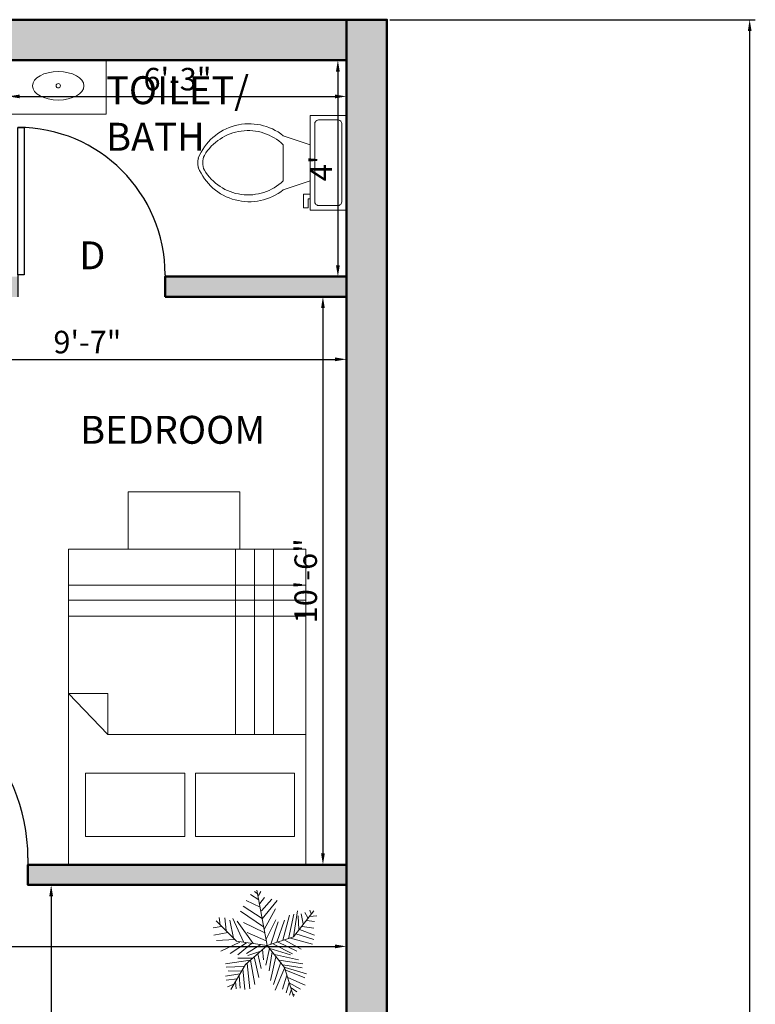
# Model space of a CAD drawing. Units: inches. Extents: x 2227 to 2709, y 1385 to 2029.
# Tile 4 of 4: x 2545 to 2709, y 1773 to 1991. Entities that reach past the tile are written whole.
import ezdxf

# ---------------------------------------------------------------- set-up
doc = ezdxf.new("R2010")
doc.units = ezdxf.units.IN
for name, color, linetype, lineweight in [('A-ANNO-DIMS', 1, 'Continuous', 18), ('A-ANNO-TEXT', 30, 'Continuous', 18), ('A-AREA-IDEN', 30, 'Continuous', 25), ('A-FLOR-FIXT', 9, 'Continuous', 18), ('A-WALL-PATT', 252, 'Continuous', 13), ('BED', 50, 'Continuous', 18), ('DOOR', 130, 'Continuous', 25), ('TREE', 80, 'Continuous', 13), ('WALL', 160, 'Continuous', 50)]:
    doc.layers.add(name, color=color, linetype=linetype, lineweight=lineweight)
doc.styles.get("Standard").update_dxf_attribs({"font": 'arial.ttf'})
doc.dimstyles.new('ISO-25', dxfattribs={"dimtxt": 5, "dimasz": 2.5, "dimexe": 1.25, "dimexo": 0.625, "dimtad": 1, "dimdec": 0, "dimlunit": 4, "dimtxsty": 'Standard', "dimcen": 2.5, "dimadec": 0, "dimazin": 0, "dimtfac": 1, "dimtdec": 0, "dimtmove": 0, "dimatfit": 3, "dimfxl": 1, "dimarcsym": 0})

# ---------------------------------------------------------------- blocks, each defined once
blk = doc.blocks.new('*U2')
for p, q in [((0, 0), (0, -6)), ((40, 0), (40, -6))]:
    blk.add_line(p, q)
blk.add_lwpolyline([(0, 0), (0, 40), (1.75, 40), (1.75, 0)], close=True)
blk.add_arc((0, 0), 40, 0, 90)
blk = doc.blocks.new('*U4')
for p, q in [((9.5, -6), (9.5, -2)), ((-10, -8.5), (-8, -8.5)), ((-10, -9.5), (-10, -8.5)), ((-8, -8.5), (-8, -8)), ((-7, -8), (-7, -9.5)), ((-4, -8), (-6, -14)), ((4, -8), (6, -14)), ((-7, -9.5), (-10, -9.5)), ((4, -14), (-4, -14))]:
    blk.add_line(p, q)
blk.add_lwpolyline([(10.5, -8), (10.5, 0), (-10.5, 0), (-10.5, -8)], close=True)
for points in [[(-9.5, -2), (-9.5, -6)], [(8.5, -1), (-8.5, -1)], [(-8.5, -7), (8.5, -7)]]:
    blk.add_lwpolyline(points)
for centre, radius, start, end in [((-8.62, -1.88), 0.884, 81.8699, 188.1301), ((8.62, -1.88), 0.884, 351.8699, 98.1301), ((-8.62, -6.12), 0.884, 171.8699, 278.1301), ((8.62, -6.12), 0.884, 261.8699, 8.1301), ((3.52, -21.58), 12.17, 141.4691, 247.9714), ((4.2, -21.82), 11.33, 136.3677, 238.9468), ((-3.52, -21.58), 12.17, 292.0284, 38.5307), ((-4.2, -21.82), 11.33, 301.053, 43.6321), ((0, -27.88), 4, 245.7318, 294.2682), ((0, -29), 4, 254.8605, 285.1395)]:
    blk.add_arc(centre, radius, start, end)
blk = doc.blocks.new('*U6')
for p, q in [((-8.737, 47.138), (-17.069, 52.711)), ((-10.186, 53.64), (-13.084, 55.962)), ((0, 0), (-10.5, 57)), ((-9.099, 51.782), (-6.563, 55.962)), ((-5.114, 28.097), (-24.676, 40.636)), ((-7.288, 39.707), (-21.778, 46.673)), ((-7.65, 43.423), (-2.578, 49.46)), ((-5.839, 35.992), (4.667, 48.067)), ((-5.114, 27.632), (10.463, 46.673)), ((-3.665, 19.273), (-27.574, 35.527)), ((-2.941, 16.486), (8.652, 37.85)), ((16.259, 5.805), (23.142, 31.348)), ((22.055, 7.198), (27.489, 32.277)), ((27, 9), (48, 36)), ((27.127, 9.056), (31.112, 35.992)), ((31.836, 30.883), (32.561, 16.486)), ((35.096, 32.741), (37.27, 22.524)), ((38.719, 34.134), (41.979, 28.561)), ((43.791, 29.954), (51.036, 30.883)), ((44.153, 36.456), (45.239, 32.741)), ((-31.5, 4.5), (-52.5, 25.5)), ((-48.585, 21.131), (-49.309, 29.026)), ((-43.513, 28.561), (-42.427, 15.558)), ((-38.442, 26.239), (-34.819, 7.663)), ((-35.544, 28.097), (-24.314, 3.947)), ((-14.533, 2.09), (-30.834, 25.31)), ((-24.314, 23.917), (-2.941, 13.7)), ((-1.129, 6.734), (9.014, 26.704)), ((3.942, 1.625), (11.187, 24.381)), ((10.101, 3.483), (17.708, 26.239)), ((40.53, 25.775), (48.862, 24.846)), ((-47.498, 19.737), (-55.83, 18.344)), ((-40.615, 13.7), (-55.105, 10.913)), ((-20.691, 13.7), (-1.129, 4.876)), ((29.662, 12.307), (48.137, 6.269)), ((33.285, 16.486), (48.862, 10.913)), ((36.183, 19.737), (48.137, 17.88)), ((-33.37, 6.269), (-52.207, 5.34)), ((-28.299, 3.483), (-47.86, -5.805)), ((-21.416, 3.018), (-38.079, -8.128)), ((0, 0), (-31.5, 4.5)), ((-15.982, 2.09), (-30.11, -9.521)), ((0, 0), (-22.5, -19.5)), ((-6.563, 1.161), (-21.416, -8.128)), ((0, 0), (27, 9)), ((0, 0), (18, -22.5)), ((6.478, 1.625), (26.04, -8.592)), ((11.187, 3.483), (30.749, -5.805)), ((18.07, 5.805), (35.096, -3.483)), ((24.229, 7.663), (46.688, 1.625)), ((-6.563, -5.805), (-19.967, -9.985)), ((-9.461, -8.592), (-6.201, -23.453)), ((-4.752, -3.483), (-3.665, -14.629)), ((2.493, -3.019), (-1.491, -20.202)), ((1.769, -2.555), (24.229, -9.521)), ((5.029, -6.27), (2.131, -25.775)), ((7.565, -9.056), (32.198, -14.629)), ((-17.431, -15.094), (-42.789, -18.809)), ((-22.5, -19.5), (-37.5, -45)), ((-15.257, -12.772), (-30.11, -12.772)), ((-20.691, -18.345), (-17.793, -44.352)), ((-17.069, -15.094), (-12.721, -40.172)), ((-13.446, -11.378), (-8.737, -32.741)), ((9.014, -11.378), (3.58, -35.992)), ((14.085, -16.951), (6.478, -40.172)), ((12.274, -15.094), (36.907, -18.809)), ((16.259, -19.738), (36.183, -22.989)), ((-28.299, -29.026), (-42.789, -31.348)), ((-24.314, -21.596), (-42.427, -22.06)), ((-26.849, -26.24), (-40.253, -25.775)), ((-25.038, -23.918), (-22.865, -45.281)), ((18.07, -22.524), (8.289, -45.745)), ((20.244, -30.419), (15.897, -44.816)), ((18, -22.5), (27, -52.5)), ((18.433, -22.524), (40.53, -29.026)), ((19.157, -25.311), (38.719, -33.206)), ((-30.834, -34.135), (-42.427, -35.528)), ((-34.457, -39.708), (-40.978, -42.494)), ((-32.646, -36.921), (-31.921, -44.352)), ((-29.023, -30.884), (-27.936, -43.887)), ((22.78, -37.85), (19.519, -48.532)), ((21.331, -32.741), (39.081, -40.636)), ((22.78, -38.314), (34.372, -44.816)), ((24.591, -45.745), (23.142, -50.854)), ((24.591, -43.423), (30.749, -47.603)), ((26.764, -49.925), (28.213, -50.854))]:
    blk.add_line(p, q)
blk = doc.blocks.new('*D13')
at = {"layer": 'A-ANNO-DIMS', "color": 0, "lineweight": -2, "transparency": 16777216}
for p, q in [((2542.71, 1981.71), (2542.71, 1973.06)), ((2617.71, 1981.71), (2617.71, 1973.06)), ((2545.21, 1974.31), (2615.21, 1974.31))]:
    blk.add_line(p, q, dxfattribs=at)
at = {"layer": 'A-ANNO-DIMS', "color": 0, "lineweight": 100, "transparency": 16777216}
for points in [[(2545.21, 1974.72), (2545.21, 1973.89), (2542.71, 1974.31)], [(2615.21, 1974.72), (2615.21, 1973.89), (2617.71, 1974.31)]]:
    blk.add_solid(points, dxfattribs=at)
at = {"layer": 'Defpoints', "color": 0, "lineweight": 100, "transparency": 16777216}
for p in [(2542.71, 1982.33), (2617.71, 1982.33), (2617.71, 1974.31)]:
    blk.add_point(p, dxfattribs=at)
at = {"layer": 'A-ANNO-DIMS', "color": 0, "transparency": 16777216, "insert": (2580.21, 1977.49), "char_height": 5, "attachment_point": 5}
blk.add_mtext('6\'-3"', dxfattribs=at)
blk = doc.blocks.new('*D14')
at = {"layer": 'A-ANNO-DIMS', "color": 0, "lineweight": -2, "transparency": 16777216}
for p, q in [((2617.09, 1982.33), (2614.58, 1982.33)), ((2615.83, 1979.83), (2615.83, 1936.83)), ((2617.09, 1934.33), (2614.58, 1934.33))]:
    blk.add_line(p, q, dxfattribs=at)
at = {"layer": 'A-ANNO-DIMS', "color": 0, "lineweight": 100, "transparency": 16777216}
for points in [[(2615.41, 1979.83), (2616.25, 1979.83), (2615.83, 1982.33)], [(2615.41, 1936.83), (2616.25, 1936.83), (2615.83, 1934.33)]]:
    blk.add_solid(points, dxfattribs=at)
at = {"layer": 'Defpoints', "color": 0, "lineweight": 100, "transparency": 16777216}
for p in [(2617.71, 1982.33), (2615.83, 1934.33), (2617.71, 1934.33)]:
    blk.add_point(p, dxfattribs=at)
at = {"layer": 'A-ANNO-DIMS', "color": 0, "transparency": 16777216, "insert": (2612.71, 1958.33), "char_height": 5, "attachment_point": 5, "rotation": 90}
blk.add_mtext("4'", dxfattribs=at)
blk = doc.blocks.new('*D15')
at = {"layer": 'A-ANNO-DIMS', "color": 0, "lineweight": -2, "transparency": 16777216}
for p, q in [((2617.09, 1929.83), (2611.26, 1929.83)), ((2612.51, 1927.33), (2612.51, 1806.33)), ((2617.09, 1803.83), (2611.26, 1803.83))]:
    blk.add_line(p, q, dxfattribs=at)
at = {"layer": 'A-ANNO-DIMS', "color": 0, "lineweight": 100, "transparency": 16777216}
for points in [[(2612.1, 1927.33), (2612.93, 1927.33), (2612.51, 1929.83)], [(2612.1, 1806.33), (2612.93, 1806.33), (2612.51, 1803.83)]]:
    blk.add_solid(points, dxfattribs=at)
at = {"layer": 'Defpoints', "color": 0, "lineweight": 100, "transparency": 16777216}
for p in [(2617.71, 1929.83), (2612.51, 1803.83), (2617.71, 1803.83)]:
    blk.add_point(p, dxfattribs=at)
at = {"layer": 'A-ANNO-DIMS', "color": 0, "transparency": 16777216, "insert": (2609.34, 1866.83), "char_height": 5, "attachment_point": 5, "rotation": 90}
blk.add_mtext('10\'-6"', dxfattribs=at)
blk = doc.blocks.new('*D16')
at = {"layer": 'A-ANNO-DIMS', "color": 0, "lineweight": -2, "transparency": 16777216}
for p, q in [((2502.71, 1804.46), (2502.71, 1917.22)), ((2617.71, 1804.46), (2617.71, 1917.22)), ((2505.21, 1915.97), (2615.21, 1915.97))]:
    blk.add_line(p, q, dxfattribs=at)
at = {"layer": 'A-ANNO-DIMS', "color": 0, "lineweight": 100, "transparency": 16777216}
for points in [[(2505.21, 1916.39), (2505.21, 1915.56), (2502.71, 1915.97)], [(2615.21, 1916.39), (2615.21, 1915.56), (2617.71, 1915.97)]]:
    blk.add_solid(points, dxfattribs=at)
at = {"layer": 'Defpoints', "color": 0, "lineweight": 100, "transparency": 16777216}
for p in [(2617.71, 1915.97), (2502.71, 1803.83), (2617.71, 1803.83)]:
    blk.add_point(p, dxfattribs=at)
at = {"layer": 'A-ANNO-DIMS', "color": 0, "transparency": 16777216, "insert": (2560.21, 1919.15), "char_height": 5, "attachment_point": 5}
blk.add_mtext('9\'-7"', dxfattribs=at)
blk = doc.blocks.new('*D29')
at = {"layer": 'A-ANNO-DIMS', "color": 0, "lineweight": -2, "transparency": 16777216}
for p, q in [((2447.21, 1798.71), (2447.21, 1784.46)), ((2617.71, 1798.71), (2617.71, 1784.46)), ((2449.71, 1785.71), (2615.21, 1785.71))]:
    blk.add_line(p, q, dxfattribs=at)
at = {"layer": 'A-ANNO-DIMS', "color": 0, "lineweight": 100, "transparency": 16777216}
for points in [[(2449.71, 1786.12), (2449.71, 1785.29), (2447.21, 1785.71)], [(2615.21, 1786.12), (2615.21, 1785.29), (2617.71, 1785.71)]]:
    blk.add_solid(points, dxfattribs=at)
at = {"layer": 'Defpoints', "color": 0, "lineweight": 100, "transparency": 16777216}
for p in [(2447.21, 1799.33), (2617.71, 1799.33), (2617.71, 1785.71)]:
    blk.add_point(p, dxfattribs=at)
at = {"layer": 'A-ANNO-DIMS', "color": 0, "transparency": 16777216, "insert": (2532.46, 1788.89), "char_height": 5, "attachment_point": 5}
blk.add_mtext('14\'-3"', dxfattribs=at)
blk = doc.blocks.new('*D30')
at = {"layer": 'A-ANNO-DIMS', "color": 0, "lineweight": -2, "transparency": 16777216}
for p, q in [((2617.09, 1799.33), (2550.92, 1799.33)), ((2552.17, 1796.83), (2552.17, 1604.83)), ((2617.09, 1602.33), (2550.92, 1602.33))]:
    blk.add_line(p, q, dxfattribs=at)
at = {"layer": 'A-ANNO-DIMS', "color": 0, "lineweight": 100, "transparency": 16777216}
for points in [[(2551.76, 1796.83), (2552.59, 1796.83), (2552.17, 1799.33)], [(2551.76, 1604.83), (2552.59, 1604.83), (2552.17, 1602.33)]]:
    blk.add_solid(points, dxfattribs=at)
at = {"layer": 'Defpoints', "color": 0, "lineweight": 100, "transparency": 16777216}
for p in [(2617.71, 1799.33), (2552.17, 1602.33), (2617.71, 1602.33)]:
    blk.add_point(p, dxfattribs=at)
at = {"layer": 'A-ANNO-DIMS', "color": 0, "transparency": 16777216, "insert": (2548.99, 1700.83), "char_height": 5, "attachment_point": 5, "rotation": 90}
blk.add_mtext('16\'-5"', dxfattribs=at)
blk = doc.blocks.new('BED-DOUBLE')
for p, q in [((37.96, 0), (28.86, -8.71)), ((37.96, -8.71), (37.96, 0)), ((55.17, -52.67), (55.17, 0)), ((58.68, -52.67), (58.68, 0)), ((62.04, -52.67), (62.04, 0)), ((28.86, -52.67), (28.86, -8.71)), ((28.86, -8.71), (37.96, -8.71)), ((28.86, -37.1), (70.02, -37.1)), ((28.86, -41.31), (70.02, -41.31)), ((28.86, -45.51), (70.02, -45.51))]:
    blk.add_line(p, q)
for points in [[(0, 0), (70.02, 0), (70.02, -52.67), (0, -52.67)], [(6.26, -25.79), (20.3, -25.79), (20.3, -3.78), (6.26, -3.78)], [(70.02, -38), (82.72, -38), (82.72, -13.23), (70.02, -13.23)], [(6.26, -50.18), (20.3, -50.18), (20.3, -28.17), (6.26, -28.17)]]:
    blk.add_lwpolyline(points, close=True)
blk = doc.blocks.new('*D48')
at = {"layer": 'A-ANNO-DIMS', "color": 0, "lineweight": -2, "transparency": 16777216}
for p, q in [((2627.34, 1991.33), (2708.51, 1991.33)), ((2707.26, 1417.83), (2707.26, 1988.83)), ((2627.34, 1415.33), (2708.51, 1415.33))]:
    blk.add_line(p, q, dxfattribs=at)
at = {"layer": 'A-ANNO-DIMS', "color": 0, "lineweight": 100, "transparency": 16777216}
for points in [[(2706.85, 1988.83), (2707.68, 1988.83), (2707.26, 1991.33)], [(2706.85, 1417.83), (2707.68, 1417.83), (2707.26, 1415.33)]]:
    blk.add_solid(points, dxfattribs=at)
at = {"layer": 'Defpoints', "color": 0, "lineweight": 100, "transparency": 16777216}
for p in [(2626.71, 1991.33), (2707.26, 1991.33), (2626.71, 1415.33)]:
    blk.add_point(p, dxfattribs=at)
at = {"layer": 'A-ANNO-DIMS', "color": 0, "transparency": 16777216, "insert": (2704.09, 1703.33), "char_height": 5, "attachment_point": 5, "rotation": 90}
blk.add_mtext('48\'-0"', dxfattribs=at)

msp = doc.modelspace()

# ---------------------------------------------------------------- hatches: boundary and pattern name
at = {"layer": 'A-WALL-PATT'}
h = msp.add_hatch(color=256, dxfattribs=at)
h.dxf.hatch_style = 1
h.paths.add_polyline_path([(2538.21, 1991.33), (2290.71, 1991.33), (2290.71, 1982.33), (2299.71, 1982.33), (2538.21, 1982.33)])
h.paths.add_polyline_path([(2299.71, 1982.33), (2290.71, 1982.33), (2290.71, 1424.33), (2299.71, 1424.33)])
h.paths.add_polyline_path([(2347.13, 1424.33), (2290.71, 1424.33), (2290.71, 1415.33), (2347.13, 1415.33)])
h.paths.add_polyline_path([(2447.21, 1424.33), (2402.93, 1424.33), (2402.93, 1415.33), (2447.21, 1415.33)])
h.paths.add_polyline_path([(2447.21, 1597.83), (2442.71, 1597.83), (2442.71, 1424.33), (2447.21, 1424.33)])
h.paths.add_polyline_path([(2396.41, 1528.83), (2299.71, 1528.83), (2299.71, 1524.33), (2396.41, 1524.33)])
h.paths.add_polyline_path([(2442.71, 1528.83), (2436.41, 1528.83), (2436.41, 1524.33), (2442.71, 1524.33)])
h.paths.add_polyline_path([(2345.64, 1667.33), (2299.71, 1667.33), (2299.71, 1662.83), (2345.64, 1662.83)])
h.paths.add_polyline_path([(2447.21, 1747.77), (2442.71, 1747.77), (2442.71, 1662.83), (2447.21, 1662.83)])
h.paths.add_polyline_path([(2442.71, 1667.33), (2401.29, 1667.33), (2401.29, 1662.83), (2442.71, 1662.83)])
h.paths.add_polyline_path([(2447.21, 1803.83), (2299.71, 1803.83), (2299.71, 1799.33), (2447.21, 1799.33)])
h.paths.add_polyline_path([(2447.21, 1799.33), (2442.71, 1799.33), (2442.71, 1787.77), (2447.21, 1787.77)])
h.paths.add_polyline_path([(2394.45, 1851.83), (2389.95, 1851.83), (2389.95, 1803.83), (2394.45, 1803.83)])
h.paths.add_polyline_path([(2327.17, 1851.83), (2322.67, 1851.83), (2322.67, 1840.2), (2327.17, 1840.2)])
h.paths.add_polyline_path([(2327.17, 1815.42), (2322.67, 1815.42), (2322.67, 1803.83), (2327.17, 1803.83)])
h.paths.add_polyline_path([(2397.41, 1856.33), (2299.71, 1856.33), (2299.71, 1851.83), (2397.41, 1851.83)])
h.paths.add_polyline_path([(2447.21, 1856.33), (2437.41, 1856.33), (2437.41, 1851.83), (2447.21, 1851.83)])
h.paths.add_polyline_path([(2447.21, 1934.33), (2442.71, 1934.33), (2442.71, 1856.33), (2447.21, 1856.33)])
h.paths.add_polyline_path([(2459.62, 1856.33), (2447.21, 1856.33), (2447.21, 1851.83), (2459.62, 1851.83)])
h.paths.add_polyline_path([(2498.21, 1856.33), (2494.53, 1856.33), (2494.53, 1851.83), (2498.21, 1851.83)])
h.paths.add_polyline_path([(2462.23, 1934.33), (2447.21, 1934.33), (2447.21, 1929.83), (2462.23, 1929.83)])
h.paths.add_polyline_path([(2507.32, 1934.33), (2483.3, 1934.33), (2483.3, 1929.83), (2507.32, 1929.83)])
h.paths.add_polyline_path([(2542.71, 1947.66), (2538.21, 1947.66), (2538.21, 1934.33), (2542.71, 1934.33)])
h.paths.add_polyline_path([(2544.78, 1934.33), (2536.35, 1934.33), (2536.35, 1929.83), (2544.78, 1929.83)])
h.paths.add_polyline_path([(2542.71, 1982.33), (2538.21, 1982.33), (2538.21, 1971.57), (2542.71, 1971.57)])
h.paths.add_polyline_path([(2346.6, 1815.57), (2382.82, 1815.57), (2382.82, 1838.66), (2346.6, 1838.66)], flags=9)
h.paths.add_polyline_path([(2457.86, 1902.08), (2494.08, 1902.08), (2494.08, 1925.17), (2457.86, 1925.17)], flags=9)
h.paths.add_polyline_path([(2500.39, 1690.49), (2545.31, 1690.49), (2545.31, 1713.58), (2500.39, 1713.58)], flags=9)
h.paths.add_polyline_path([(2528.08, 1476.92), (2562.42, 1476.92), (2562.42, 1489.69), (2528.08, 1489.69)], flags=9)
h.paths.add_polyline_path([(2349.07, 1476.93), (2390.15, 1476.93), (2390.15, 1489.69), (2349.07, 1489.69)], flags=9)
h.paths.add_polyline_path([(2347.99, 1586.39), (2381.37, 1586.39), (2381.37, 1609.48), (2347.99, 1609.48)], flags=9)
h.paths.add_polyline_path([(2328.07, 1742.46), (2375.88, 1742.46), (2375.88, 1755.23), (2328.07, 1755.23)], flags=9)
h.paths.add_polyline_path([(2556.42, 1893.75), (2604.23, 1893.75), (2604.23, 1906.51), (2556.42, 1906.51)], flags=9)
h.paths.add_polyline_path([(2323.02, 1893.88), (2370.83, 1893.88), (2370.83, 1906.64), (2323.02, 1906.64)], flags=9)
h.paths.add_polyline_path([(2562.19, 1958.77), (2598.41, 1958.77), (2598.41, 1981.86), (2562.19, 1981.86)], flags=9)
h.paths.add_polyline_path([(2482.23, 1953.14), (2507.92, 1953.14), (2507.92, 1965.9), (2482.23, 1965.9)], flags=9)
h = msp.add_hatch(color=256, dxfattribs=at)
h.dxf.hatch_style = 1
h.paths.add_polyline_path([(2617.71, 1991.33), (2538.21, 1991.33), (2538.21, 1982.33), (2617.71, 1982.33)])
h.paths.add_polyline_path([(2626.71, 1991.33), (2617.71, 1991.33), (2617.71, 1982.33), (2617.71, 1415.33), (2626.71, 1415.33)])
h.paths.add_polyline_path([(2617.71, 1934.33), (2577.48, 1934.33), (2577.48, 1929.83), (2617.71, 1929.83)])
h.paths.add_polyline_path([(2502.71, 1929.83), (2498.21, 1929.83), (2498.21, 1803.83), (2502.71, 1803.83)])
h.paths.add_polyline_path([(2617.71, 1803.83), (2547.01, 1803.83), (2547.01, 1799.33), (2617.71, 1799.33)])
h.paths.add_polyline_path([(2507.01, 1803.83), (2498.21, 1803.83), (2498.21, 1799.33), (2507.01, 1799.33)])
h.paths.add_polyline_path([(2617.71, 1602.33), (2607.17, 1602.33), (2607.17, 1601.18), (2607.17, 1597.83), (2617.71, 1597.83)])

# ---------------------------------------------------------------- linework, layer by layer
at = {"layer": 'A-FLOR-FIXT'}
msp.add_lwpolyline([(2542.71, 1982.33), (2564.37, 1982.33), (2564.37, 1970.37), (2542.71, 1970.37)], close=True, dxfattribs=at)
msp.add_circle((2553.75, 1976.66), 0.482, dxfattribs=at)
msp.add_ellipse((2553.75, 1976.66), major_axis=(5.71, 0), ratio=0.554218, dxfattribs=at)
at = {"layer": 'WALL'}
for p, q in [((2290.71, 1991.33), (2626.71, 1991.33)), ((2626.71, 1991.33), (2626.71, 1415.33)), ((2577.48, 1934.33), (2617.71, 1934.33)), ((2577.48, 1929.83), (2617.71, 1929.83)), ((2617.71, 1929.83), (2617.71, 1803.83)), ((2617.71, 1803.83), (2547.01, 1803.83)), ((2617.71, 1799.33), (2547.01, 1799.33)), ((2617.71, 1799.33), (2617.71, 1602.33))]:
    msp.add_line(p, q, dxfattribs=at)
for points in [[(2447.21, 1415.33), (2290.71, 1415.33), (2290.71, 1991.33), (2626.71, 1991.33), (2626.71, 1415.33), (2617.71, 1415.33)], [(2447.21, 1424.33), (2299.71, 1424.33), (2299.71, 1982.33), (2617.71, 1982.33), (2617.71, 1424.33)]]:
    msp.add_lwpolyline(points, dxfattribs=at)
for points in [[(2538.21, 1991.33), (2617.71, 1991.33), (2617.71, 1982.33), (2538.21, 1982.33)], [(2617.71, 1991.33), (2626.71, 1991.33), (2626.71, 1415.33), (2617.71, 1415.33)], [(2577.48, 1929.83), (2617.71, 1929.83), (2617.71, 1934.33), (2577.48, 1934.33)], [(2617.71, 1799.33), (2547.01, 1799.33), (2547.01, 1803.83), (2617.71, 1803.83)]]:
    msp.add_lwpolyline(points, close=True, dxfattribs=at)

# ---------------------------------------------------------------- block references
at = {"layer": 'A-FLOR-FIXT', "xscale": -1, "rotation": 270}
msp.add_blockref('*U4', (2617.71, 1959.59), dxfattribs=at)
at = {"layer": 'BED', "rotation": 89.99999999999957}
msp.add_blockref('BED-DOUBLE', (2556.03, 1803.83), dxfattribs=at)
at = {"layer": 'DOOR', "xscale": 0.8174402911474247, "yscale": 0.8174402911474247, "zscale": 0.8174402911474247}
msp.add_blockref('*U2', (2544.78, 1934.74), dxfattribs=at)
at = {"layer": 'DOOR'}
msp.add_blockref('*U2', (2507.01, 1805.33), dxfattribs=at)
at = {"layer": 'TREE', "xscale": 0.2153773147918839, "yscale": 0.2153773147918839, "zscale": 0.2153773147918839}
msp.add_blockref('*U6', (2600.13, 1785.87), dxfattribs=at)

# ---------------------------------------------------------------- texts
at = {"layer": 'A-ANNO-TEXT', "insert": (2558.41, 1942.14), "char_height": 6.19, "attachment_point": 1}
msp.add_mtext_dynamic_manual_height_columns('D', width=156.7329, gutter_width=30.97, heights=[0], dxfattribs=at)
at = {"layer": 'A-AREA-IDEN', "char_height": 6.194, "attachment_point": 1}
for s, insert in [('TOILET/\\PBATH', (2564.37, 1978.78)), ('BEDROOM', (2558.6, 1903.43))]:
    msp.add_mtext_dynamic_manual_height_columns(s, width=156.7329, gutter_width=30.97, heights=[0], dxfattribs=dict(at, insert=insert))

# ---------------------------------------------------------------- dimensions: what is measured, and where the dimension line sits
at = {"layer": 'A-ANNO-DIMS'}
for base, p1, p2, override, picture, middle in [((2707.26, 1991.33), (2626.71, 1415.33), (2626.71, 1991.33), {"dimdec": 1, "dimlfac": 1, "dimrnd": 0, "dimzin": 1, "dimdsep": 46, "dimlunit": 4, "dimfrac": 2}, '*D48', (2704.09, 1703.33)), ((2615.83, 1934.33), (2617.71, 1982.33), (2617.71, 1934.33), {"dimclrd": 0, "dimclre": 0, "dimclrt": 0}, '*D14', (2612.71, 1958.33)), ((2612.51, 1803.83), (2617.71, 1929.83), (2617.71, 1803.83), {"dimclrd": 0, "dimclre": 0, "dimclrt": 0}, '*D15', (2609.34, 1866.83)), ((2552.17, 1602.33), (2617.71, 1799.33), (2617.71, 1602.33), {"dimclrd": 0, "dimclre": 0, "dimclrt": 0}, '*D30', (2548.99, 1700.83))]:
    dim = msp.add_linear_dim(base=base, p1=p1, p2=p2, angle=90, dimstyle='ISO-25', override=override, dxfattribs=at)
    dim.commit()
    dim.dimension.update_dxf_attribs({"geometry": picture, "text_midpoint": middle})
for base, p1, p2, picture, middle in [((2617.71, 1974.31), (2542.71, 1982.33), (2617.71, 1982.33), '*D13', (2580.21, 1977.49)), ((2617.71, 1915.97), (2502.71, 1803.83), (2617.71, 1803.83), '*D16', (2560.21, 1919.15)), ((2617.71377381, 1785.70618657), (2447.21377381, 1799.33305883), (2617.71377381, 1799.33305883), '*D29', (2532.46377381, 1788.88575683))]:
    dim = msp.add_linear_dim(base=base, p1=p1, p2=p2, dimstyle='ISO-25', override={"dimclrd": 0, "dimclre": 0, "dimclrt": 0}, dxfattribs=at)
    dim.commit()
    dim.dimension.update_dxf_attribs({"geometry": picture, "text_midpoint": middle})

doc.saveas('drawing.dxf')
